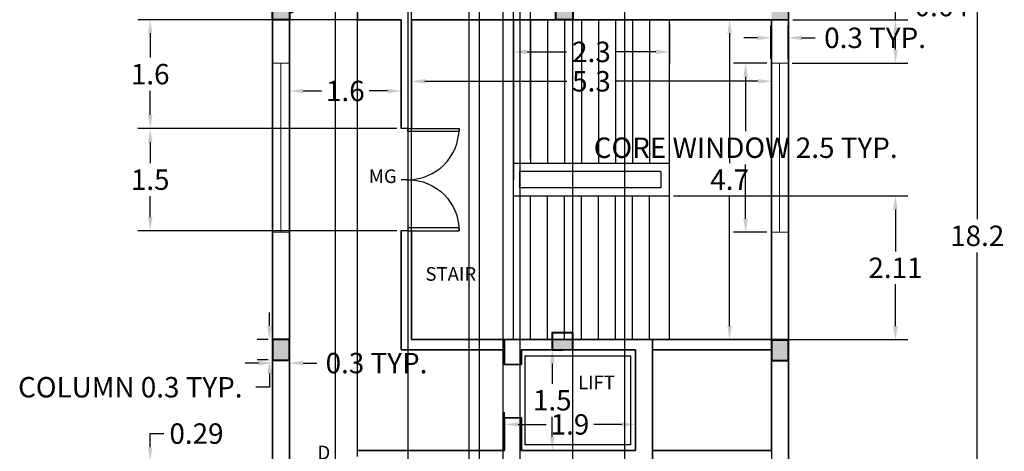
# Model space of a CAD drawing. Units: metres. Extents: x 106.5 to 121.4, y 89.1 to 111.8.
# Tile 3 of 5: x 106.5 to 121, y 97.3 to 103.6. Entities that reach past the tile are written whole.
import ezdxf

# ---------------------------------------------------------------- set-up
doc = ezdxf.new("R2010")
doc.units = ezdxf.units.M
doc.header["$MEASUREMENT"] = 0
doc.layers.get('0').update_dxf_attribs({"color": 1})
for name, color, linetype, lineweight in [('A-ANNO-DIMS', 5, 'Continuous', 18), ('A-ANNO-TEXT', 4, 'Continuous', 18), ('A-AREA-IDEN', 4, 'Continuous', 18), ('A-COLS-PATT', 18, 'Continuous', 13), ('A-FLOR-EVTR', 2, 'Continuous', 25), ('A-WALL', 1, 'Continuous', 35), ('COLUMN', 244, 'Continuous', 40), ('DR', 2, 'Continuous', 25), ('STAIR', 6, 'Continuous', 25), ('WNDW', 3, 'Continuous', 18)]:
    doc.layers.add(name, color=color, linetype=linetype, lineweight=lineweight)
doc.styles.get("Standard").update_dxf_attribs({"font": 'arial.ttf'})
doc.dimstyles.get("Standard").update_dxf_attribs({"dimtxt": 0.3, "dimasz": 0.2, "dimexe": 0.18, "dimexo": 0.0625, "dimgap": 0.09, "dimtad": 0, "dimtih": 1, "dimtoh": 1, "dimdec": 1, "dimzin": 0, "dimdsep": 46, "dimtxsty": 'Standard', "dimcen": 0.09, "dimadec": 0, "dimazin": 0, "dimtfac": 1, "dimtdec": 1, "dimtofl": 0, "dimtmove": 0, "dimatfit": 3, "dimfxl": 1, "dimtolj": 1, "dimtzin": 0, "dimarcsym": 0})

# ---------------------------------------------------------------- blocks, each defined once
blk = doc.blocks.new('*U5')
for p, q in [((0, 0), (0, -100)), ((1000, 0), (1000, -100))]:
    blk.add_line(p, q)
blk.add_lwpolyline([(0, 0), (0, 1000), (43.75, 1000), (43.75, 0)], close=True)
blk.add_arc((0, 0), 1000, 0, 90)
blk = doc.blocks.new('*U6')
for p, q in [((-750, 0), (-750, 100)), ((0, 0), (0, 100))]:
    blk.add_line(p, q)
blk.add_lwpolyline([(0, 0), (0, -750), (-43.75, -750), (-43.75, 0)], close=True)
blk.add_arc((0, 0), 750, 180, 270)
blk = doc.blocks.new('*D8')
at = {"layer": 'A-ANNO-DIMS', "color": 0, "lineweight": -2, "ltscale": 0.5, "transparency": 16777216}
for p, q in [((117.47, 103.594), (116.737, 103.594)), ((116.917, 103.394), (116.917, 101.484)), ((116.917, 99.094), (116.917, 101.004)), ((117.47, 98.894), (116.737, 98.894))]:
    blk.add_line(p, q, dxfattribs=at)
at = {"layer": 'A-ANNO-DIMS', "color": 0, "lineweight": -3, "ltscale": 0.5, "transparency": 16777216}
for points in [[(116.884, 103.394), (116.951, 103.394), (116.917, 103.594)], [(116.884, 99.094), (116.951, 99.094), (116.917, 98.894)]]:
    blk.add_solid(points, dxfattribs=at)
at = {"layer": 'Defpoints', "color": 0, "lineweight": -3, "ltscale": 0.5, "transparency": 16777216}
for p in [(117.533, 103.594), (116.917, 98.894), (117.533, 98.894)]:
    blk.add_point(p, dxfattribs=at)
at = {"layer": 'A-ANNO-DIMS', "color": 0, "ltscale": 0.5, "transparency": 16777216, "insert": (116.917, 101.244), "char_height": 0.3, "attachment_point": 5}
blk.add_mtext('\\A1;4.7', dxfattribs=at)
blk = doc.blocks.new('*D9')
at = {"layer": 'A-ANNO-DIMS', "color": 0, "lineweight": -2, "ltscale": 0.5, "transparency": 16777216}
for p, q in [((112.243, 103.531), (112.243, 102.509)), ((117.533, 103.537), (117.533, 102.509)), ((112.443, 102.689), (114.525, 102.689)), ((117.333, 102.689), (115.251, 102.689))]:
    blk.add_line(p, q, dxfattribs=at)
at = {"layer": 'A-ANNO-DIMS', "color": 0, "lineweight": -3, "ltscale": 0.5, "transparency": 16777216}
for points in [[(112.443, 102.723), (112.443, 102.656), (112.243, 102.689)], [(117.333, 102.723), (117.333, 102.656), (117.533, 102.689)]]:
    blk.add_solid(points, dxfattribs=at)
at = {"layer": 'Defpoints', "color": 0, "lineweight": -3, "ltscale": 0.5, "transparency": 16777216}
for p in [(112.243, 103.594), (117.533, 103.6), (117.533, 102.689)]:
    blk.add_point(p, dxfattribs=at)
at = {"layer": 'A-ANNO-DIMS', "color": 0, "ltscale": 0.5, "transparency": 16777216, "insert": (114.888, 102.689), "char_height": 0.3, "attachment_point": 5}
blk.add_mtext('\\A1;5.3', dxfattribs=at)
blk = doc.blocks.new('*D10')
at = {"layer": 'A-ANNO-DIMS', "color": 0, "lineweight": -2, "ltscale": 0.5, "transparency": 16777216}
for p, q in [((113.743, 103.531), (113.743, 102.941)), ((116.033, 103.531), (116.033, 102.941)), ((113.943, 103.121), (114.522, 103.121)), ((115.833, 103.121), (115.254, 103.121))]:
    blk.add_line(p, q, dxfattribs=at)
at = {"layer": 'A-ANNO-DIMS', "color": 0, "lineweight": -3, "ltscale": 0.5, "transparency": 16777216}
for points in [[(113.943, 103.155), (113.943, 103.088), (113.743, 103.121)], [(115.833, 103.155), (115.833, 103.088), (116.033, 103.121)]]:
    blk.add_solid(points, dxfattribs=at)
at = {"layer": 'Defpoints', "color": 0, "lineweight": -3, "ltscale": 0.5, "transparency": 16777216}
for p in [(113.743, 103.594), (116.033, 103.594), (116.033, 103.121)]:
    blk.add_point(p, dxfattribs=at)
at = {"layer": 'A-ANNO-DIMS', "color": 0, "ltscale": 0.5, "transparency": 16777216, "insert": (114.888, 103.121), "char_height": 0.3, "attachment_point": 5}
blk.add_mtext('\\A1;2.3', dxfattribs=at)
blk = doc.blocks.new('*D11')
at = {"layer": 'A-ANNO-DIMS', "color": 0, "lineweight": -2, "ltscale": 0.5, "transparency": 16777216}
for p, q in [((110.453, 102.731), (110.453, 102.367)), ((112.093, 102.731), (112.093, 102.367)), ((110.653, 102.547), (110.924, 102.547)), ((111.893, 102.547), (111.622, 102.547))]:
    blk.add_line(p, q, dxfattribs=at)
at = {"layer": 'A-ANNO-DIMS', "color": 0, "lineweight": -3, "ltscale": 0.5, "transparency": 16777216}
for points in [[(110.653, 102.58), (110.653, 102.513), (110.453, 102.547)], [(111.893, 102.58), (111.893, 102.513), (112.093, 102.547)]]:
    blk.add_solid(points, dxfattribs=at)
at = {"layer": 'Defpoints', "color": 0, "lineweight": -3, "ltscale": 0.5, "transparency": 16777216}
for p in [(110.453, 102.794), (112.093, 102.794), (110.453, 102.547)]:
    blk.add_point(p, dxfattribs=at)
at = {"layer": 'A-ANNO-DIMS', "color": 0, "ltscale": 0.5, "transparency": 16777216, "insert": (111.273, 102.547), "char_height": 0.3, "attachment_point": 5}
blk.add_mtext('\\A1;1.6', dxfattribs=at)
blk = doc.blocks.new('*D22')
at = {"layer": 'A-ANNO-DIMS', "color": 0, "lineweight": -2, "ltscale": 0.5, "transparency": 16777216}
for p, q in [((114.376, 98.744), (114.493, 98.744)), ((114.313, 98.544), (114.313, 98.247)), ((114.313, 97.464), (114.313, 97.761)), ((114.376, 97.264), (114.493, 97.264))]:
    blk.add_line(p, q, dxfattribs=at)
at = {"layer": 'A-ANNO-DIMS', "color": 0, "lineweight": -3, "ltscale": 0.5, "transparency": 16777216}
for points in [[(114.28, 98.544), (114.347, 98.544), (114.313, 98.744)], [(114.28, 97.464), (114.347, 97.464), (114.313, 97.264)]]:
    blk.add_solid(points, dxfattribs=at)
at = {"layer": 'Defpoints', "color": 0, "lineweight": -3, "ltscale": 0.5, "transparency": 16777216}
for p in [(114.313, 98.744), (114.313, 97.264), (114.313, 97.264)]:
    blk.add_point(p, dxfattribs=at)
at = {"layer": 'A-ANNO-DIMS', "color": 0, "ltscale": 0.5, "transparency": 16777216, "insert": (114.313, 98.004), "char_height": 0.3, "attachment_point": 5}
blk.add_mtext('\\A1;1.5', dxfattribs=at)
blk = doc.blocks.new('*D23')
at = {"layer": 'A-ANNO-DIMS', "color": 0, "lineweight": -2, "ltscale": 0.5, "transparency": 16777216}
for p, q in [((113.613, 97.566), (113.613, 97.829)), ((115.533, 97.534), (115.533, 97.829)), ((113.813, 97.649), (114.224, 97.649)), ((115.333, 97.649), (114.922, 97.649))]:
    blk.add_line(p, q, dxfattribs=at)
at = {"layer": 'A-ANNO-DIMS', "color": 0, "lineweight": -3, "ltscale": 0.5, "transparency": 16777216}
for points in [[(113.813, 97.683), (113.813, 97.616), (113.613, 97.649)], [(115.333, 97.683), (115.333, 97.616), (115.533, 97.649)]]:
    blk.add_solid(points, dxfattribs=at)
at = {"layer": 'Defpoints', "color": 0, "lineweight": -3, "ltscale": 0.5, "transparency": 16777216}
for p in [(115.533, 97.649), (113.613, 97.503), (115.533, 97.471)]:
    blk.add_point(p, dxfattribs=at)
at = {"layer": 'A-ANNO-DIMS', "color": 0, "ltscale": 0.5, "transparency": 16777216, "insert": (114.573, 97.649), "char_height": 0.3, "attachment_point": 5}
blk.add_mtext('\\A1;1.9', dxfattribs=at)
blk = doc.blocks.new('*D24')
at = {"layer": 'A-ANNO-DIMS', "color": 0, "lineweight": -2, "ltscale": 0.5, "transparency": 16777216}
for p, q in [((117.845, 109.504), (120.734, 109.504)), ((120.554, 109.304), (120.554, 100.662)), ((120.554, 91.534), (120.554, 100.176)), ((117.845, 91.334), (120.734, 91.334))]:
    blk.add_line(p, q, dxfattribs=at)
at = {"layer": 'A-ANNO-DIMS', "color": 0, "lineweight": -3, "ltscale": 0.5, "transparency": 16777216}
for points in [[(120.521, 109.304), (120.588, 109.304), (120.554, 109.504)], [(120.521, 91.534), (120.588, 91.534), (120.554, 91.334)]]:
    blk.add_solid(points, dxfattribs=at)
at = {"layer": 'Defpoints', "color": 0, "lineweight": -3, "ltscale": 0.5, "transparency": 16777216}
for p in [(117.783, 109.504), (117.782, 91.334), (120.554, 91.334)]:
    blk.add_point(p, dxfattribs=at)
at = {"layer": 'A-ANNO-DIMS', "color": 0, "ltscale": 0.5, "transparency": 16777216, "insert": (120.554, 100.419), "char_height": 0.3, "attachment_point": 5}
blk.add_mtext('\\A1;18.2', dxfattribs=at)
blk = doc.blocks.new('WIN-2484-CORE')
at = {"ltscale": 0.5}
blk.add_line((0.125, 2.484), (0.125, 0), dxfattribs=at)
blk.add_lwpolyline([(0, 2.484), (0.25, 2.484), (0.25, 0), (0, 0)], close=True, dxfattribs=at)
blk = doc.blocks.new('COL-250X300')
at = {"ltscale": 0.5}
blk.add_lwpolyline([(0, 0.3), (0.25, 0.3), (0.25, 0), (0, 0)], close=True, dxfattribs=at)
blk = doc.blocks.new('*D36')
at = {"layer": 'A-ANNO-DIMS', "color": 0, "lineweight": -2, "ltscale": 0.5, "transparency": 16777216}
for p, q in [((110.158, 99.095), (110.158, 99.295)), ((110.14, 98.895), (109.978, 98.895)), ((110.14, 98.595), (109.978, 98.595)), ((110.158, 98.395), (110.158, 98.195)), ((110.158, 98.195), (109.958, 98.195))]:
    blk.add_line(p, q, dxfattribs=at)
at = {"layer": 'A-ANNO-DIMS', "color": 0, "lineweight": -3, "ltscale": 0.5, "transparency": 16777216}
for points in [[(110.125, 99.095), (110.191, 99.095), (110.158, 98.895)], [(110.125, 98.395), (110.191, 98.395), (110.158, 98.595)]]:
    blk.add_solid(points, dxfattribs=at)
at = {"layer": 'Defpoints', "color": 0, "lineweight": -3, "ltscale": 0.5, "transparency": 16777216}
for p in [(110.203, 98.895), (110.158, 98.595), (110.203, 98.595)]:
    blk.add_point(p, dxfattribs=at)
at = {"layer": 'A-ANNO-DIMS', "color": 0, "ltscale": 0.5, "transparency": 16777216, "insert": (108.115, 98.195), "char_height": 0.3, "attachment_point": 5}
blk.add_mtext('\\A1;COLUMN 0.3 TYP.', dxfattribs=at)
blk = doc.blocks.new('*D37')
at = {"layer": 'A-ANNO-DIMS', "color": 0, "lineweight": -2, "ltscale": 0.5, "transparency": 16777216}
for p, q in [((110.003, 98.55), (109.803, 98.55)), ((110.203, 98.532), (110.203, 98.37)), ((110.453, 98.532), (110.453, 98.37)), ((110.653, 98.55), (110.853, 98.55))]:
    blk.add_line(p, q, dxfattribs=at)
at = {"layer": 'A-ANNO-DIMS', "color": 0, "lineweight": -3, "ltscale": 0.5, "transparency": 16777216}
for points in [[(110.003, 98.583), (110.003, 98.516), (110.203, 98.55)], [(110.653, 98.583), (110.653, 98.516), (110.453, 98.55)]]:
    blk.add_solid(points, dxfattribs=at)
at = {"layer": 'Defpoints', "color": 0, "lineweight": -3, "ltscale": 0.5, "transparency": 16777216}
for p in [(110.203, 98.595), (110.453, 98.595), (110.453, 98.55)]:
    blk.add_point(p, dxfattribs=at)
at = {"layer": 'A-ANNO-DIMS', "color": 0, "ltscale": 0.5, "transparency": 16777216, "insert": (111.731, 98.55), "char_height": 0.3, "attachment_point": 5}
blk.add_mtext('\\A1;0.3 TYP.', dxfattribs=at)
blk = doc.blocks.new('*D42')
at = {"layer": 'A-ANNO-DIMS', "color": 0, "lineweight": -2, "ltscale": 0.5, "transparency": 16777216}
for p, q in [((117.463, 102.955), (116.973, 102.955)), ((117.153, 102.755), (117.153, 101.958)), ((117.153, 100.671), (117.153, 101.468)), ((117.463, 100.471), (116.973, 100.471))]:
    blk.add_line(p, q, dxfattribs=at)
at = {"layer": 'A-ANNO-DIMS', "color": 0, "lineweight": -3, "ltscale": 0.5, "transparency": 16777216}
for points in [[(117.119, 102.755), (117.186, 102.755), (117.153, 102.955)], [(117.119, 100.671), (117.186, 100.671), (117.153, 100.471)]]:
    blk.add_solid(points, dxfattribs=at)
at = {"layer": 'Defpoints', "color": 0, "lineweight": -3, "ltscale": 0.5, "transparency": 16777216}
for p in [(117.153, 102.955), (117.525, 102.955), (117.525, 100.471)]:
    blk.add_point(p, dxfattribs=at)
at = {"layer": 'A-ANNO-DIMS', "color": 0, "ltscale": 0.5, "transparency": 16777216, "insert": (117.153, 101.713), "char_height": 0.3, "attachment_point": 5}
blk.add_mtext('\\A1;CORE WINDOW 2.5 TYP.', dxfattribs=at)
blk = doc.blocks.new('*D43')
at = {"layer": 'A-ANNO-DIMS', "color": 0, "lineweight": -2, "ltscale": 0.5, "transparency": 16777216}
for p, q in [((117.525, 103.017), (117.525, 103.507)), ((117.775, 103.017), (117.775, 103.507)), ((117.325, 103.327), (117.125, 103.327)), ((117.975, 103.327), (118.175, 103.327))]:
    blk.add_line(p, q, dxfattribs=at)
at = {"layer": 'A-ANNO-DIMS', "color": 0, "lineweight": -3, "ltscale": 0.5, "transparency": 16777216}
for points in [[(117.325, 103.361), (117.325, 103.294), (117.525, 103.327)], [(117.975, 103.361), (117.975, 103.294), (117.775, 103.327)]]:
    blk.add_solid(points, dxfattribs=at)
at = {"layer": 'Defpoints', "color": 0, "lineweight": -3, "ltscale": 0.5, "transparency": 16777216}
for p in [(117.775, 103.327), (117.525, 102.955), (117.775, 102.955)]:
    blk.add_point(p, dxfattribs=at)
at = {"layer": 'A-ANNO-DIMS', "color": 0, "ltscale": 0.5, "transparency": 16777216, "insert": (119.054, 103.327), "char_height": 0.3, "attachment_point": 5}
blk.add_mtext('\\A1;0.3 TYP.', dxfattribs=at)
blk = doc.blocks.new('*D50')
at = {"layer": 'A-ANNO-DIMS', "color": 0, "lineweight": -2, "ltscale": 0.5, "transparency": 16777216}
for p, q in [((118.331, 97.006), (118.654, 97.006)), ((118.474, 96.806), (118.474, 96.564)), ((118.474, 95.833), (118.474, 96.074)), ((118.331, 95.633), (118.654, 95.633))]:
    blk.add_line(p, q, dxfattribs=at)
at = {"layer": 'A-ANNO-DIMS', "color": 0, "lineweight": -3, "ltscale": 0.5, "transparency": 16777216}
for points in [[(118.441, 96.806), (118.508, 96.806), (118.474, 97.006)], [(118.441, 95.833), (118.508, 95.833), (118.474, 95.633)]]:
    blk.add_solid(points, dxfattribs=at)
at = {"layer": 'Defpoints', "color": 0, "lineweight": -3, "ltscale": 0.5, "transparency": 16777216}
for p in [(118.268, 97.006), (118.474, 97.006), (118.268, 95.633)]:
    blk.add_point(p, dxfattribs=at)
at = {"layer": 'A-ANNO-DIMS', "color": 0, "ltscale": 0.5, "transparency": 16777216, "insert": (118.474, 96.319), "char_height": 0.3, "attachment_point": 5}
blk.add_mtext('\\A1;SIDE LINTEL 1.4 TYP.', dxfattribs=at)
blk = doc.blocks.new('*D58')
at = {"layer": 'A-ANNO-DIMS', "color": 0, "lineweight": -2, "ltscale": 0.5, "transparency": 16777216}
for p, q in [((110.453, 97.206), (110.453, 111.769)), ((111.453, 97.176), (111.453, 111.769)), ((110.253, 111.589), (110.053, 111.589)), ((111.653, 111.589), (111.853, 111.589))]:
    blk.add_line(p, q, dxfattribs=at)
at = {"layer": 'A-ANNO-DIMS', "color": 0, "lineweight": -3, "ltscale": 0.5, "transparency": 16777216}
for points in [[(110.253, 111.622), (110.253, 111.555), (110.453, 111.589)], [(111.653, 111.622), (111.653, 111.555), (111.453, 111.589)]]:
    blk.add_solid(points, dxfattribs=at)
at = {"layer": 'Defpoints', "color": 0, "lineweight": -3, "ltscale": 0.5, "transparency": 16777216}
for p in [(111.453, 111.589), (110.453, 97.144), (111.453, 97.114)]:
    blk.add_point(p, dxfattribs=at)
at = {"layer": 'A-ANNO-DIMS', "color": 0, "ltscale": 0.5, "transparency": 16777216, "insert": (110.953, 111.589), "char_height": 0.3, "attachment_point": 5}
blk.add_mtext('\\A1;1.0', dxfattribs=at)
blk = doc.blocks.new('*D59')
at = {"layer": 'A-ANNO-DIMS', "color": 0, "lineweight": -2, "ltscale": 0.5, "transparency": 16777216}
for p, q in [((112.194, 94.346), (112.194, 111.769)), ((113.093, 94.346), (113.093, 111.769)), ((112.394, 111.589), (112.893, 111.589)), ((113.093, 111.589), (113.293, 111.589))]:
    blk.add_line(p, q, dxfattribs=at)
at = {"layer": 'A-ANNO-DIMS', "color": 0, "lineweight": -3, "ltscale": 0.5, "transparency": 16777216}
for points in [[(112.394, 111.622), (112.394, 111.555), (112.194, 111.589)], [(112.893, 111.622), (112.893, 111.555), (113.093, 111.589)]]:
    blk.add_solid(points, dxfattribs=at)
at = {"layer": 'Defpoints', "color": 0, "lineweight": -3, "ltscale": 0.5, "transparency": 16777216}
for p in [(113.093, 111.589), (112.194, 94.284), (113.093, 94.284)]:
    blk.add_point(p, dxfattribs=at)
at = {"layer": 'A-ANNO-DIMS', "color": 0, "ltscale": 0.5, "transparency": 16777216, "insert": (113.772, 111.589), "char_height": 0.3, "attachment_point": 5}
blk.add_mtext('\\A1;0.90', dxfattribs=at)
blk = doc.blocks.new('*D60')
at = {"layer": 'A-ANNO-DIMS', "color": 0, "lineweight": -2, "ltscale": 0.5, "transparency": 16777216}
for p, q in [((113.243, 94.086), (113.243, 111.769)), ((113.841, 94.086), (113.841, 111.769)), ((113.443, 111.589), (113.641, 111.589)), ((113.841, 111.589), (114.041, 111.589))]:
    blk.add_line(p, q, dxfattribs=at)
at = {"layer": 'A-ANNO-DIMS', "color": 0, "lineweight": -3, "ltscale": 0.5, "transparency": 16777216}
for points in [[(113.443, 111.622), (113.443, 111.555), (113.243, 111.589)], [(113.641, 111.622), (113.641, 111.555), (113.841, 111.589)]]:
    blk.add_solid(points, dxfattribs=at)
at = {"layer": 'Defpoints', "color": 0, "lineweight": -3, "ltscale": 0.5, "transparency": 16777216}
for p in [(113.841, 111.589), (113.243, 94.024), (113.841, 94.024)]:
    blk.add_point(p, dxfattribs=at)
at = {"layer": 'A-ANNO-DIMS', "color": 0, "ltscale": 0.5, "transparency": 16777216, "insert": (114.637, 111.589), "char_height": 0.3, "attachment_point": 5}
blk.add_mtext('\\A1;0.598', dxfattribs=at)
blk = doc.blocks.new('*D63')
at = {"layer": 'A-ANNO-DIMS', "color": 0, "lineweight": -2, "ltscale": 0.5, "transparency": 16777216}
for p, q in [((110.453, 91.646), (110.453, 111.769)), ((111.127, 91.646), (111.127, 111.769)), ((110.653, 111.589), (110.927, 111.589)), ((111.127, 111.589), (111.327, 111.589))]:
    blk.add_line(p, q, dxfattribs=at)
at = {"layer": 'A-ANNO-DIMS', "color": 0, "lineweight": -3, "ltscale": 0.5, "transparency": 16777216}
for points in [[(110.653, 111.622), (110.653, 111.555), (110.453, 111.589)], [(110.927, 111.622), (110.927, 111.555), (111.127, 111.589)]]:
    blk.add_solid(points, dxfattribs=at)
at = {"layer": 'Defpoints', "color": 0, "lineweight": -3, "ltscale": 0.5, "transparency": 16777216}
for p in [(111.127, 111.589), (110.453, 91.584), (111.127, 91.584)]:
    blk.add_point(p, dxfattribs=at)
at = {"layer": 'A-ANNO-DIMS', "color": 0, "ltscale": 0.5, "transparency": 16777216, "insert": (111.806, 111.589), "char_height": 0.3, "attachment_point": 5}
blk.add_mtext('\\A1;0.67', dxfattribs=at)
blk = doc.blocks.new('*D64')
at = {"layer": 'A-ANNO-DIMS', "color": 0, "lineweight": -2, "ltscale": 0.5, "transparency": 16777216}
for p, q in [((113.243, 91.646), (113.243, 111.769)), ((113.591, 91.646), (113.591, 111.769)), ((113.043, 111.589), (112.843, 111.589)), ((113.791, 111.589), (113.991, 111.589))]:
    blk.add_line(p, q, dxfattribs=at)
at = {"layer": 'A-ANNO-DIMS', "color": 0, "lineweight": -3, "ltscale": 0.5, "transparency": 16777216}
for points in [[(113.043, 111.622), (113.043, 111.555), (113.243, 111.589)], [(113.791, 111.622), (113.791, 111.555), (113.591, 111.589)]]:
    blk.add_solid(points, dxfattribs=at)
at = {"layer": 'Defpoints', "color": 0, "lineweight": -3, "ltscale": 0.5, "transparency": 16777216}
for p in [(113.591, 111.589), (113.243, 91.584), (113.591, 91.584)]:
    blk.add_point(p, dxfattribs=at)
at = {"layer": 'A-ANNO-DIMS', "color": 0, "ltscale": 0.5, "transparency": 16777216, "insert": (114.471, 111.589), "char_height": 0.3, "attachment_point": 5}
blk.add_mtext('\\A1;0.35', dxfattribs=at)
blk = doc.blocks.new('*D65')
at = {"layer": 'A-ANNO-DIMS', "color": 0, "lineweight": -2, "ltscale": 0.5, "transparency": 16777216}
for p, q in [((114.613, 91.646), (114.613, 111.769)), ((115.379, 91.646), (115.379, 111.769)), ((114.813, 111.589), (115.179, 111.589)), ((115.379, 111.589), (115.579, 111.589))]:
    blk.add_line(p, q, dxfattribs=at)
at = {"layer": 'A-ANNO-DIMS', "color": 0, "lineweight": -3, "ltscale": 0.5, "transparency": 16777216}
for points in [[(114.813, 111.622), (114.813, 111.555), (114.613, 111.589)], [(115.179, 111.622), (115.179, 111.555), (115.379, 111.589)]]:
    blk.add_solid(points, dxfattribs=at)
at = {"layer": 'Defpoints', "color": 0, "lineweight": -3, "ltscale": 0.5, "transparency": 16777216}
for p in [(115.379, 111.589), (114.613, 91.584), (115.379, 91.584)]:
    blk.add_point(p, dxfattribs=at)
at = {"layer": 'A-ANNO-DIMS', "color": 0, "ltscale": 0.5, "transparency": 16777216, "insert": (116.175, 111.589), "char_height": 0.3, "attachment_point": 5}
blk.add_mtext('\\A1;0.766', dxfattribs=at)
blk = doc.blocks.new('*D69')
at = {"layer": 'A-ANNO-DIMS', "color": 0, "lineweight": -2, "ltscale": 0.5, "transparency": 16777216}
for p, q in [((108.407, 97.314), (108.407, 97.514)), ((108.407, 97.514), (108.607, 97.514)), ((117.47, 97.114), (108.227, 97.114)), ((117.47, 96.819), (108.227, 96.819)), ((108.407, 96.619), (108.407, 96.419))]:
    blk.add_line(p, q, dxfattribs=at)
at = {"layer": 'A-ANNO-DIMS', "color": 0, "lineweight": -3, "ltscale": 0.5, "transparency": 16777216}
for points in [[(108.374, 97.314), (108.441, 97.314), (108.407, 97.114)], [(108.374, 96.619), (108.441, 96.619), (108.407, 96.819)]]:
    blk.add_solid(points, dxfattribs=at)
at = {"layer": 'Defpoints', "color": 0, "lineweight": -3, "ltscale": 0.5, "transparency": 16777216}
for p in [(108.407, 97.114), (117.533, 97.114), (117.532, 96.819)]:
    blk.add_point(p, dxfattribs=at)
at = {"layer": 'A-ANNO-DIMS', "color": 0, "ltscale": 0.5, "transparency": 16777216, "insert": (109.087, 97.514), "char_height": 0.3, "attachment_point": 5}
blk.add_mtext('\\A1;0.29', dxfattribs=at)
blk = doc.blocks.new('*D71')
at = {"layer": 'A-ANNO-DIMS', "color": 0, "lineweight": -2, "ltscale": 0.5, "transparency": 16777216}
for p, q in [((112.03, 101.994), (108.227, 101.994)), ((108.407, 101.794), (108.407, 101.487)), ((108.407, 100.694), (108.407, 101.001)), ((112.03, 100.494), (108.227, 100.494))]:
    blk.add_line(p, q, dxfattribs=at)
at = {"layer": 'A-ANNO-DIMS', "color": 0, "lineweight": -3, "ltscale": 0.5, "transparency": 16777216}
for points in [[(108.374, 101.794), (108.441, 101.794), (108.407, 101.994)], [(108.374, 100.694), (108.441, 100.694), (108.407, 100.494)]]:
    blk.add_solid(points, dxfattribs=at)
at = {"layer": 'Defpoints', "color": 0, "lineweight": -3, "ltscale": 0.5, "transparency": 16777216}
for p in [(108.407, 101.994), (112.093, 101.994), (112.093, 100.494)]:
    blk.add_point(p, dxfattribs=at)
at = {"layer": 'A-ANNO-DIMS', "color": 0, "ltscale": 0.5, "transparency": 16777216, "insert": (108.407, 101.244), "char_height": 0.3, "attachment_point": 5}
blk.add_mtext('\\A1;1.5', dxfattribs=at)
blk = doc.blocks.new('*D72')
at = {"layer": 'A-ANNO-DIMS', "color": 0, "lineweight": -2, "ltscale": 0.5, "transparency": 16777216}
for p, q in [((112.243, 98.956), (112.243, 111.769)), ((113.743, 98.956), (113.743, 111.769)), ((112.443, 111.589), (112.643, 111.589)), ((113.543, 111.589), (113.343, 111.589))]:
    blk.add_line(p, q, dxfattribs=at)
at = {"layer": 'A-ANNO-DIMS', "color": 0, "lineweight": -3, "ltscale": 0.5, "transparency": 16777216}
for points in [[(112.443, 111.622), (112.443, 111.555), (112.243, 111.589)], [(113.543, 111.622), (113.543, 111.555), (113.743, 111.589)]]:
    blk.add_solid(points, dxfattribs=at)
at = {"layer": 'Defpoints', "color": 0, "lineweight": -3, "ltscale": 0.5, "transparency": 16777216}
for p in [(113.743, 111.589), (112.243, 98.894), (113.743, 98.894)]:
    blk.add_point(p, dxfattribs=at)
at = {"layer": 'A-ANNO-DIMS', "color": 0, "ltscale": 0.5, "transparency": 16777216, "insert": (112.993, 111.589), "char_height": 0.3, "attachment_point": 5}
blk.add_mtext('\\A1;1.5', dxfattribs=at)
blk = doc.blocks.new('*D73')
at = {"layer": 'A-ANNO-DIMS', "color": 0, "lineweight": -2, "ltscale": 0.5, "transparency": 16777216}
for p, q in [((116.095, 101.004), (119.533, 101.004)), ((119.353, 100.804), (119.353, 100.189)), ((119.353, 99.094), (119.353, 99.708)), ((116.095, 98.894), (119.533, 98.894))]:
    blk.add_line(p, q, dxfattribs=at)
at = {"layer": 'A-ANNO-DIMS', "color": 0, "lineweight": -3, "ltscale": 0.5, "transparency": 16777216}
for points in [[(119.32, 100.804), (119.387, 100.804), (119.353, 101.004)], [(119.32, 99.094), (119.387, 99.094), (119.353, 98.894)]]:
    blk.add_solid(points, dxfattribs=at)
at = {"layer": 'Defpoints', "color": 0, "lineweight": -3, "ltscale": 0.5, "transparency": 16777216}
for p in [(116.033, 101.004), (119.353, 101.004), (116.033, 98.894)]:
    blk.add_point(p, dxfattribs=at)
at = {"layer": 'A-ANNO-DIMS', "color": 0, "ltscale": 0.5, "transparency": 16777216, "insert": (119.353, 99.949), "char_height": 0.3, "attachment_point": 5}
blk.add_mtext('\\A1;2.11', dxfattribs=at)
blk = doc.blocks.new('*D74')
at = {"layer": 'A-ANNO-DIMS', "color": 0, "lineweight": -2, "ltscale": 0.5, "transparency": 16777216}
for p, q in [((115.783, 98.681), (115.783, 89.069)), ((117.533, 98.681), (117.533, 89.069)), ((115.983, 89.249), (116.191, 89.249)), ((117.333, 89.249), (117.125, 89.249))]:
    blk.add_line(p, q, dxfattribs=at)
at = {"layer": 'A-ANNO-DIMS', "color": 0, "lineweight": -3, "ltscale": 0.5, "transparency": 16777216}
for points in [[(115.983, 89.282), (115.983, 89.215), (115.783, 89.249)], [(117.333, 89.282), (117.333, 89.215), (117.533, 89.249)]]:
    blk.add_solid(points, dxfattribs=at)
at = {"layer": 'Defpoints', "color": 0, "lineweight": -3, "ltscale": 0.5, "transparency": 16777216}
for p in [(115.783, 98.744), (117.533, 98.744), (117.533, 89.249)]:
    blk.add_point(p, dxfattribs=at)
at = {"layer": 'A-ANNO-DIMS', "color": 0, "ltscale": 0.5, "transparency": 16777216, "insert": (116.658, 89.249), "char_height": 0.3, "attachment_point": 5}
blk.add_mtext('\\A1;1.75', dxfattribs=at)
blk = doc.blocks.new('*D75')
at = {"layer": 'A-ANNO-DIMS', "color": 0, "lineweight": -2, "ltscale": 0.5, "transparency": 16777216}
for p, q in [((119.353, 103.594), (119.353, 103.794)), ((119.353, 103.794), (119.553, 103.794)), ((117.845, 103.594), (119.533, 103.594)), ((119.353, 103.155), (119.353, 103.394)), ((117.838, 102.955), (119.533, 102.955))]:
    blk.add_line(p, q, dxfattribs=at)
at = {"layer": 'A-ANNO-DIMS', "color": 0, "lineweight": -3, "ltscale": 0.5, "transparency": 16777216}
for points in [[(119.32, 103.394), (119.387, 103.394), (119.353, 103.594)], [(119.32, 103.155), (119.387, 103.155), (119.353, 102.955)]]:
    blk.add_solid(points, dxfattribs=at)
at = {"layer": 'Defpoints', "color": 0, "lineweight": -3, "ltscale": 0.5, "transparency": 16777216}
for p in [(117.783, 103.594), (119.353, 103.594), (117.775, 102.955)]:
    blk.add_point(p, dxfattribs=at)
at = {"layer": 'A-ANNO-DIMS', "color": 0, "ltscale": 0.5, "transparency": 16777216, "insert": (120.032, 103.794), "char_height": 0.3, "attachment_point": 5}
blk.add_mtext('\\A1;0.64', dxfattribs=at)
blk = doc.blocks.new('*D76')
at = {"layer": 'A-ANNO-DIMS', "color": 0, "lineweight": -2, "ltscale": 0.5, "transparency": 16777216}
for p, q in [((113.743, 101.546), (113.743, 111.769)), ((113.993, 101.546), (113.993, 111.769)), ((113.543, 111.589), (113.343, 111.589)), ((114.193, 111.589), (114.393, 111.589))]:
    blk.add_line(p, q, dxfattribs=at)
at = {"layer": 'A-ANNO-DIMS', "color": 0, "lineweight": -3, "ltscale": 0.5, "transparency": 16777216}
for points in [[(113.543, 111.622), (113.543, 111.555), (113.743, 111.589)], [(114.193, 111.622), (114.193, 111.555), (113.993, 111.589)]]:
    blk.add_solid(points, dxfattribs=at)
at = {"layer": 'Defpoints', "color": 0, "lineweight": -3, "ltscale": 0.5, "transparency": 16777216}
for p in [(113.993, 111.589), (113.743, 101.484), (113.993, 101.484)]:
    blk.add_point(p, dxfattribs=at)
at = {"layer": 'A-ANNO-DIMS', "color": 0, "ltscale": 0.5, "transparency": 16777216, "insert": (114.874, 111.589), "char_height": 0.3, "attachment_point": 5}
blk.add_mtext('\\A1;0.25', dxfattribs=at)
blk = doc.blocks.new('*D77')
at = {"layer": 'A-ANNO-DIMS', "color": 0, "lineweight": -2, "ltscale": 0.5, "transparency": 16777216}
for p, q in [((112.03, 103.594), (108.227, 103.594)), ((108.407, 103.394), (108.407, 103.037)), ((108.407, 102.194), (108.407, 102.551)), ((112.03, 101.994), (108.227, 101.994))]:
    blk.add_line(p, q, dxfattribs=at)
at = {"layer": 'A-ANNO-DIMS', "color": 0, "lineweight": -3, "ltscale": 0.5, "transparency": 16777216}
for points in [[(108.374, 103.394), (108.441, 103.394), (108.407, 103.594)], [(108.374, 102.194), (108.441, 102.194), (108.407, 101.994)]]:
    blk.add_solid(points, dxfattribs=at)
at = {"layer": 'Defpoints', "color": 0, "lineweight": -3, "ltscale": 0.5, "transparency": 16777216}
for p in [(108.407, 103.594), (112.093, 103.594), (112.093, 101.994)]:
    blk.add_point(p, dxfattribs=at)
at = {"layer": 'A-ANNO-DIMS', "color": 0, "ltscale": 0.5, "transparency": 16777216, "insert": (108.407, 102.794), "char_height": 0.3, "attachment_point": 5}
blk.add_mtext('\\A1;1.6', dxfattribs=at)

msp = doc.modelspace()

# ---------------------------------------------------------------- hatches: boundary and pattern name
at = {"layer": 'A-COLS-PATT', "ltscale": 0.5}
h = msp.add_hatch(color=256, dxfattribs=at)
h.dxf.hatch_style = 1
h.paths.add_polyline_path([(110.4529, 103.8929), (110.2029, 103.8929), (110.2029, 103.5938), (110.4529, 103.5938)])
h.paths.add_polyline_path([(114.4629, 103.8938), (114.3632, 103.8938), (114.3632, 103.7438), (114.4629, 103.7438)])
h.paths.add_polyline_path([(114.6129, 103.8938), (114.4629, 103.8938), (114.4629, 103.7438), (114.6129, 103.7438)])
h.paths.add_polyline_path([(114.6132, 103.7438), (114.4629, 103.7438), (114.3632, 103.7438), (114.3632, 103.5938), (114.6132, 103.5938)])
h.paths.add_polyline_path([(117.7829, 103.8996), (117.5329, 103.8996), (117.5329, 103.5996), (117.7829, 103.5996)])
h.paths.add_polyline_path([(117.7829, 98.888), (117.5329, 98.888), (117.5329, 98.588), (117.7829, 98.588)])
h.paths.add_polyline_path([(110.4529, 98.8938), (110.2029, 98.8938), (110.2029, 98.5947), (110.4529, 98.5947)])
h.paths.add_polyline_path([(114.6132, 98.8938), (114.3132, 98.8938), (114.3132, 98.7438), (114.4632, 98.7438), (114.6132, 98.7438)])
h.paths.add_polyline_path([(110.4529, 91.6338), (110.2029, 91.6338), (110.2029, 91.3338), (110.4529, 91.3338)])
h.paths.add_polyline_path([(114.6132, 91.5838), (114.6129, 91.5838), (114.6129, 91.6338), (114.4629, 91.6338), (114.4629, 91.5838), (114.3632, 91.5838), (114.3632, 91.3338), (114.6132, 91.3338)])
h.paths.add_polyline_path([(117.7821, 91.6338), (117.5329, 91.6338), (117.5329, 91.5838), (117.5321, 91.3338), (117.7821, 91.3338)])

# ---------------------------------------------------------------- linework, layer by layer
at = {"layer": 'A-FLOR-EVTR', "ltscale": 0.5}
msp.add_lwpolyline([(113.9165, 98.6545), (115.4637, 98.6545), (115.4637, 97.3482), (113.9165, 97.3482)], close=True, dxfattribs=at)
at = {"layer": 'A-WALL'}
for p, q in [((110.2029, 109.5038), (110.2029, 101.3638)), ((117.7829, 101.3638), (117.7829, 109.5038)), ((110.4529, 103.5938), (110.2029, 103.5938)), ((110.4529, 103.5938), (110.4529, 101.3638)), ((110.4529, 98.8938), (110.4529, 103.5929)), ((112.0929, 103.5938), (111.4529, 103.5938)), ((112.0929, 103.5938), (112.0929, 101.9938)), ((117.7829, 103.5938), (112.2429, 103.5938)), ((112.2429, 103.5938), (112.2429, 101.9938)), ((117.5329, 101.3638), (117.5329, 103.5938)), ((117.5329, 103.5938), (117.5329, 98.8938)), ((110.2029, 91.3338), (110.2029, 101.9438)), ((117.7829, 101.9438), (117.7829, 91.3338)), ((112.0929, 98.7438), (112.0929, 100.4938)), ((112.2429, 98.8938), (112.2429, 100.4938)), ((110.4529, 98.8938), (110.2029, 98.8938)), ((117.7829, 98.8938), (112.2429, 98.8938)), ((113.6129, 98.5274), (113.6129, 98.8938)), ((115.7829, 98.8938), (115.7829, 97.1137)), ((113.6129, 98.7438), (112.0929, 98.7438)), ((114.6129, 98.7438), (113.8629, 98.7438)), ((113.8629, 98.5274), (113.8629, 98.7438)), ((115.5329, 98.7438), (114.6129, 98.7438)), ((115.5329, 98.7438), (115.5329, 97.2637)), ((117.5329, 98.7438), (115.7829, 98.7438)), ((110.4529, 94.4338), (110.4529, 98.5947)), ((117.5329, 98.588), (117.5329, 97.2637)), ((113.6129, 97.2637), (113.6129, 97.7431)), ((113.8629, 97.2637), (113.8629, 97.7431)), ((113.6129, 97.2637), (111.4517, 97.2637)), ((114.6129, 97.2637), (113.8629, 97.2637)), ((115.5329, 97.2637), (114.6129, 97.2637)), ((117.5329, 97.2637), (115.7829, 97.2637))]:
    msp.add_line(p, q, dxfattribs=at)
at = {"layer": 'A-WALL', "ltscale": 0.5}
for p, q in [((113.8629, 98.5274), (113.6129, 98.5274)), ((113.8629, 97.7431), (113.6129, 97.7431))]:
    msp.add_line(p, q, dxfattribs=at)
at = {"layer": 'COLUMN', "ltscale": 0.5}
msp.add_lwpolyline([(114.6132, 98.7438), (114.6132, 98.9938), (114.3132, 98.9938), (114.3132, 98.7438), (114.4632, 98.7438)], dxfattribs=at)
at = {"layer": 'STAIR'}
for p, q in [((113.7429, 103.5938), (113.7429, 101.2438)), ((113.9929, 103.5938), (113.9929, 101.4838)), ((114.2429, 103.5938), (114.2429, 101.4838)), ((114.4929, 103.5938), (114.4929, 101.4838)), ((114.7429, 103.5938), (114.7429, 101.4838)), ((114.9929, 103.5938), (114.9929, 101.4838)), ((115.2429, 103.5938), (115.2429, 101.4838)), ((115.4929, 103.5938), (115.4929, 101.4838)), ((115.7429, 103.5938), (115.7429, 101.4838)), ((116.0329, 98.8938), (116.0329, 103.5938)), ((116.0329, 101.4838), (113.7429, 101.4838)), ((113.7429, 98.8938), (113.7429, 101.2438)), ((115.9073, 101.3638), (113.8298, 101.3638)), ((115.9073, 101.1238), (113.8298, 101.1238)), ((116.0329, 101.0038), (113.7429, 101.0038)), ((113.9929, 98.8938), (113.9929, 101.0038)), ((114.2429, 98.8938), (114.2429, 101.0038)), ((114.4929, 98.8938), (114.4929, 101.0038)), ((114.7429, 98.8938), (114.7429, 101.0038)), ((114.9929, 98.8938), (114.9929, 101.0038)), ((115.2429, 98.8938), (115.2429, 101.0038)), ((115.4929, 98.8938), (115.4929, 101.0038)), ((115.7429, 98.8938), (115.7429, 101.0038))]:
    msp.add_line(p, q, dxfattribs=at)
at = {"layer": 'STAIR', "ltscale": 0.5}
for p, q in [((113.8298, 101.3638), (113.8298, 101.1238)), ((115.9073, 101.3638), (115.9073, 101.1238))]:
    msp.add_line(p, q, dxfattribs=at)

# ---------------------------------------------------------------- block references
at = {"layer": 'COLUMN'}
for p in [(110.203, 103.593), (114.3633, 103.5939)]:
    msp.add_blockref('COL-250X300', p, dxfattribs=at)
at = {"layer": 'COLUMN', "extrusion": (0, 0, -1), "zscale": -1, "rotation": 180}
for p in [(-110.203, 98.8946), (-117.533, 98.888)]:
    msp.add_blockref('COL-250X300', p, dxfattribs=at)
at = {"layer": 'DR', "xscale": 0.001, "yscale": 0.001, "zscale": 0.001}
msp.add_blockref('*U5', (110.4529, 103.6938), dxfattribs=at)
at = {"layer": 'DR', "yscale": 0.001, "zscale": 0.001}
for p, xscale, rotation in [((112.1929, 101.9938), 0.001, 90), ((112.1929, 100.4938), -0.001, 90.00000000000152)]:
    msp.add_blockref('*U6', p, dxfattribs=dict(at, xscale=xscale, rotation=rotation))
at = {"layer": 'WNDW'}
for p in [(110.203, 100.471), (117.5255, 100.471)]:
    msp.add_blockref('WIN-2484-CORE', p, dxfattribs=at)

# ---------------------------------------------------------------- texts
at = {"layer": 'A-ANNO-TEXT', "ltscale": 0.5, "char_height": 0.2, "attachment_point": 1}
for s, insert in [('MG', (111.6181, 101.3943)), ('D', (110.8641, 97.3364))]:
    msp.add_mtext_dynamic_manual_height_columns(s, width=0.320447, gutter_width=1, heights=[0], dxfattribs=dict(at, insert=insert))
at = {"layer": 'A-AREA-IDEN', "ltscale": 0.5, "char_height": 0.2, "attachment_point": 1}
for s, width, insert in [('STAIR ', 0.439121, (112.4498, 99.9592)), ('LIFT', 0.773551, (114.6901, 98.3646))]:
    msp.add_mtext_dynamic_manual_height_columns(s, width=width, gutter_width=1, heights=[0], dxfattribs=dict(at, insert=insert))

# ---------------------------------------------------------------- dimensions: what is measured, and where the dimension line sits
at = {"layer": 'A-ANNO-DIMS', "ltscale": 0.5}
for base, p1, p2, override, picture, middle in [((111.4529, 111.5888), (110.4529, 97.1438), (111.4529, 97.1137), {"dimdec": 1, "dimlfac": 1, "dimrnd": 0, "dimzin": 0, "dimdsep": 46, "dimlunit": 2}, '*D58', (110.9529, 111.5888)), ((111.1267, 111.5888), (110.4529, 91.5838), (111.1267, 91.5838), {"dimdec": 2, "dimlfac": 1, "dimrnd": 0, "dimzin": 0, "dimdsep": 46, "dimlunit": 2}, '*D63', (111.8063, 111.5888)), ((113.0929, 111.5888), (112.1943, 94.2838), (113.0929, 94.2838), {"dimdec": 2, "dimlfac": 1, "dimrnd": 0, "dimzin": 0, "dimdsep": 46, "dimlunit": 2}, '*D59', (113.772, 111.5888)), ((113.7429, 111.5888), (112.2429, 98.8938), (113.7429, 98.8938), {"dimdec": 1, "dimlfac": 1, "dimrnd": 0, "dimzin": 0, "dimdsep": 46, "dimlunit": 2}, '*D72', (112.9929, 111.5888)), ((113.5905, 111.5888), (113.2429, 91.5838), (113.5905, 91.5838), {"dimdec": 2, "dimlfac": 1, "dimrnd": 0, "dimzin": 0, "dimdsep": 46, "dimlunit": 2}, '*D64', (114.4713, 111.5888)), ((113.8408, 111.5888), (113.2429, 94.0238), (113.8408, 94.0238), {"dimdec": 3, "dimlfac": 1, "dimrnd": 0, "dimzin": 0, "dimdsep": 46, "dimlunit": 2}, '*D60', (114.6373, 111.5888)), ((113.9929, 111.5888), (113.7429, 101.4838), (113.9929, 101.4838), {"dimdec": 2, "dimlfac": 1, "dimrnd": 0, "dimzin": 0, "dimdsep": 46, "dimlunit": 2}, '*D76', (114.8737, 111.5888)), ((115.3789, 111.5888), (114.6129, 91.5838), (115.3789, 91.5838), {"dimdec": 3, "dimlfac": 1, "dimrnd": 0, "dimzin": 0, "dimdsep": 46, "dimlunit": 2}, '*D65', (116.1749, 111.5888)), ((117.5329, 102.6893), (112.2429, 103.5938), (117.5329, 103.5996), {"dimclrd": 0, "dimclre": 0, "dimclrt": 0}, '*D9', (114.8879, 102.6893)), ((116.0329, 103.1212), (113.7429, 103.5938), (116.0329, 103.5938), {"dimclrd": 0, "dimclre": 0, "dimclrt": 0}, '*D10', (114.8879, 103.1212)), ((110.4529, 102.5467), (112.0929, 102.7938), (110.4529, 102.7938), {"dimclrd": 0, "dimclre": 0, "dimclrt": 0}, '*D11', (111.2729, 102.5467)), ((117.5329, 89.2488), (115.7829, 98.7438), (117.5329, 98.7438), {"dimdec": 2, "dimlfac": 1, "dimrnd": 0, "dimzin": 0, "dimdsep": 46, "dimlunit": 2}, '*D74', (116.6579, 89.2488)), ((115.5329, 97.6493), (113.6129, 97.5034), (115.5329, 97.471), {"dimclrd": 0, "dimclre": 0, "dimclrt": 0}, '*D23', (114.5729, 97.6493))]:
    dim = msp.add_linear_dim(base=base, p1=p1, p2=p2, dimstyle='Standard', override=override, dxfattribs=at)
    dim.commit()
    dim.dimension.update_dxf_attribs({"geometry": picture, "text_midpoint": middle})
for base, p1, p2, override, picture, middle in [((120.5543, 91.3338), (117.7829, 109.5038), (117.7821, 91.3338), {"dimclrd": 0, "dimclre": 0, "dimclrt": 0}, '*D24', (120.5543, 100.4188)), ((119.3535, 103.5938), (117.7754, 102.9546), (117.7829, 103.5938), {"dimdec": 2, "dimlfac": 1, "dimrnd": 0, "dimzin": 0, "dimdsep": 46, "dimlunit": 2}, '*D75', (120.0325, 103.7938)), ((108.4073, 103.5938), (112.0929, 101.9938), (112.0929, 103.5938), {"dimdec": 1, "dimlfac": 1, "dimrnd": 0, "dimzin": 0, "dimdsep": 46, "dimlunit": 2}, '*D77', (108.4073, 102.7938)), ((116.9172, 98.8938), (117.5329, 103.5938), (117.5329, 98.8938), {"dimclrd": 0, "dimclre": 0, "dimclrt": 0}, '*D8', (116.9172, 101.2438)), ((108.4073, 101.9938), (112.0929, 100.4938), (112.0929, 101.9938), {"dimdec": 1, "dimlfac": 1, "dimrnd": 0, "dimzin": 0, "dimdsep": 46, "dimlunit": 2}, '*D71', (108.4073, 101.2438)), ((119.3535, 101.0038), (116.0329, 98.8938), (116.0329, 101.0038), {"dimdec": 2, "dimlfac": 1, "dimrnd": 0, "dimzin": 0, "dimdsep": 46, "dimlunit": 2}, '*D73', (119.3535, 99.9488)), ((114.3132, 97.2637), (114.3132, 98.7438), (114.3132, 97.2637), {"dimclrd": 0, "dimclre": 0, "dimclrt": 0}, '*D22', (114.3132, 98.0037)), ((108.4073, 97.1137), (117.5322, 96.8191), (117.5329, 97.1137), {"dimdec": 2, "dimlfac": 1, "dimrnd": 0, "dimzin": 0, "dimdsep": 46, "dimlunit": 2}, '*D69', (109.0872, 97.5137))]:
    dim = msp.add_linear_dim(base=base, p1=p1, p2=p2, angle=90, dimstyle='Standard', override=override, dxfattribs=at)
    dim.commit()
    dim.dimension.update_dxf_attribs({"geometry": picture, "text_midpoint": middle})
for base, p1, p2, picture, middle in [((117.7753725261, 103.327206493), (117.5253725261, 102.9546403061), (117.7753725261, 102.9546403061), '*D43', (119.0537422396, 103.327206493)), ((110.4529178957, 98.5496680935), (110.2029178957, 98.5946680935), (110.4529178957, 98.5946680935), '*D37', (111.7312876092, 98.5496680935))]:
    dim = msp.add_linear_dim(base=base, p1=p1, p2=p2, text='<> TYP.', dimstyle='Standard', override={"dimdec": 1, "dimlfac": 1, "dimrnd": 0, "dimzin": 0, "dimdsep": 46, "dimlunit": 2}, dxfattribs=at)
    dim.commit()
    dim.dimension.update_dxf_attribs({"geometry": picture, "text_midpoint": middle})
for base, p1, p2, angle, text, picture, middle in [((117.1528, 102.9546), (117.5254, 100.4709), (117.5254, 102.9546), 90, 'CORE WINDOW <> TYP.', '*D42', (117.1528, 101.7128)), ((110.1579, 98.5947), (110.2029, 98.8947), (110.2029, 98.5947), 270, 'COLUMN <> TYP.', '*D36', (108.115, 98.1947)), ((118.4744, 97.0058), (118.2685, 95.6327), (118.2685, 97.0058), 90, 'SIDE LINTEL <> TYP.', '*D50', (118.4744, 96.3193))]:
    dim = msp.add_linear_dim(base=base, p1=p1, p2=p2, angle=angle, text=text, dimstyle='Standard', override={"dimdec": 1, "dimlfac": 1, "dimrnd": 0, "dimzin": 0, "dimdsep": 46, "dimlunit": 2}, dxfattribs=at)
    dim.commit()
    dim.dimension.update_dxf_attribs({"geometry": picture, "text_midpoint": middle})

doc.saveas('drawing.dxf')
